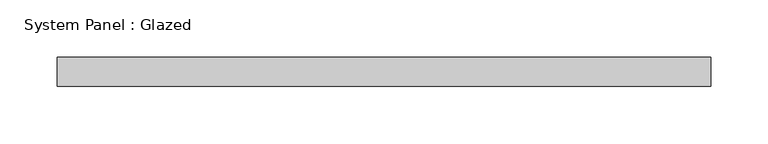
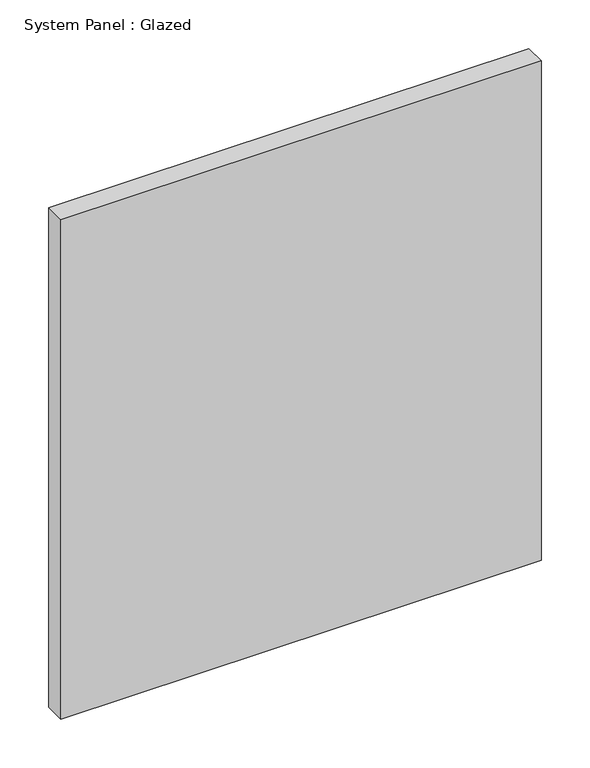
"""IFC4 building model written with IfcOpenShell, lengths in millimetres: plate geometry, System Panel : Glazed."""

from ifc_helpers import new_model, si_unit, origin, origin_with_axes, place, context, project, spatial, polyline, outline, extrude, source, transform, mapped, element, save


def system_panel_glazed_f02c31ce(model_context):
    return source(origin(), model_context, "Body", "SweptSolid", [
        extrude(outline(polyline([(285.75, 19.05), (-285.75, 19.05), (-285.75, 44.45), (285.75, 44.45), (285.75, 19.05)])), origin_with_axes(), (0.0, 0.0, 1.0), 628.65),
    ])


if __name__ == "__main__":
    model = new_model("IFC4")
    model_context = context("Model", 3, world=origin())
    ifc_project = project(units=[si_unit("LENGTHUNIT", "METRE", prefix="MILLI")], contexts=[model_context])
    site = spatial("IfcSite", under=ifc_project)
    building = spatial("IfcBuilding", under=site)
    placement = place(None, origin())
    system_panel_glazed_shape = system_panel_glazed_f02c31ce(model_context)
    element("IfcPlate", 1, ObjectType="System Panel : Glazed", at=placement, inside=building, context=model_context, shape_type="MappedRepresentation", body=[
        mapped(system_panel_glazed_shape, transform((0.0, 0.0, 0.0), x_axis=(1.0, 0.0, 0.0), y_axis=(0.0, 1.0, 0.0), z_axis=(0.0, 0.0, 1.0))),
    ])
    save(model, "model.ifc")

# Revit data of these elements
# Type "System Panel : Glazed"
#   Construction Type Id = "GSP4R"
#   Analytic Construction = "1/8 in Pilkington single glazing"
#   Visual Light Transmittance = 0.9
#   Solar Heat Gain Coefficient = 0.86
#   Heat Transfer Coefficient (U) = 1.18115 BTU/(h·ft²·°F)
#   Define Thermal Properties by = 1
# Element 1 (IfcPlate, "System Panel : Glazed")
#   Materials on its faces: "Glass"
# Materials
#   "Glass": class "Glass", colour RGB 0 128 192, transparency 0.75, Description = "Soda Lime Glass", Cost = 0
